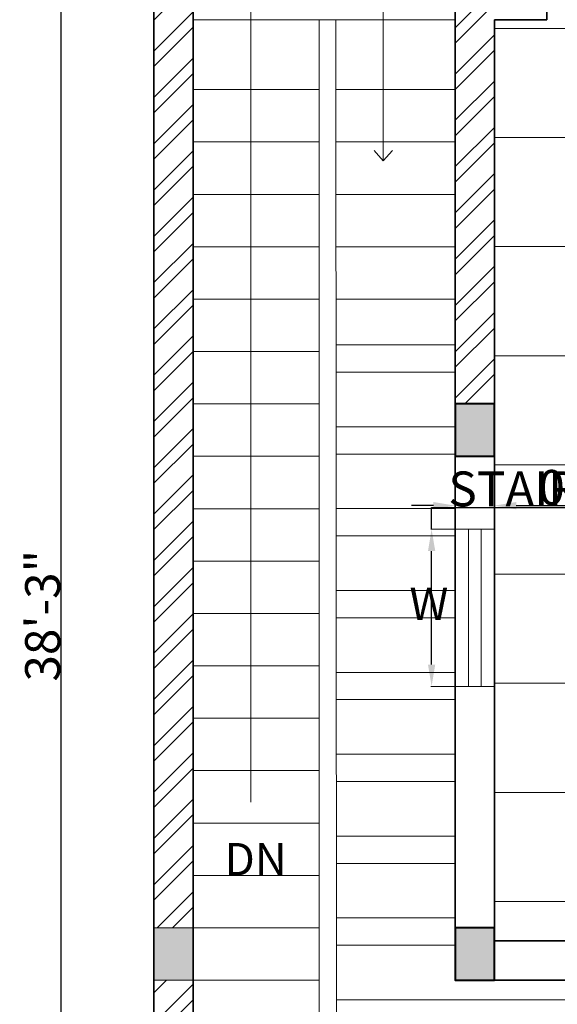
# Model space of a CAD drawing. Units: inches. Extents: x 351 to 1738, y -265 to 286.
# Tile 21 of 38: x 1004 to 1127, y -63 to 163. Entities that reach past the tile are written whole.
import ezdxf

# ---------------------------------------------------------------- set-up
doc = ezdxf.new("R2010")
doc.units = ezdxf.units.IN
doc.header["$MEASUREMENT"] = 0
for name, color, linetype, lineweight in [('A-ANNO-DIMS', 2, 'Continuous', 18), ('A-ANNO-SYMB', 7, 'Continuous', 18), ('A-COLS', 7, 'Continuous', 40), ('A-COLS-PATT', 6, 'Continuous', 13), ('A-FLOR-PATT', 9, 'Continuous', 9), ('A-FLOR-STRS', 7, 'Continuous', 18), ('A-GLAZ', 4, 'Continuous', 18), ('A-WALL', 7, 'Continuous', 35), ('A-WALL-PATT', 152, 'Continuous', 13)]:
    doc.layers.add(name, color=color, linetype=linetype, lineweight=lineweight)
doc.styles.add('Annotative', font='arial.ttf')
doc.styles.get("Standard").update_dxf_attribs({"font": 'arial.ttf'})
doc.dimstyles.get("Standard").update_dxf_attribs({"dimtxt": 8, "dimasz": 5, "dimexe": 0.18, "dimexo": 0.0625, "dimgap": 0.09, "dimtad": 1, "dimtoh": 1, "dimzin": 0, "dimdsep": 46, "dimlunit": 4, "dimtxsty": 'Standard', "dimcen": 0, "dimclre": 256, "dimadec": 0, "dimazin": 0, "dimtfac": 1, "dimtofl": 0, "dimtmove": 0, "dimatfit": 3, "dimfxl": 1, "dimtolj": 1, "dimtzin": 0, "dimlwe": -1, "dimarcsym": 0})

# ---------------------------------------------------------------- blocks, each defined once
blk = doc.blocks.new('*D8')
at = {"layer": 'A-ANNO-DIMS', "color": 0, "transparency": 16777216}
for p, q in [((1034.64, 255.96), (1013.22, 255.96)), ((1034.64, -203.04), (1013.22, -203.04))]:
    blk.add_line(p, q, dxfattribs=at)
at = {"layer": 'A-ANNO-DIMS', "color": 0, "lineweight": -2, "transparency": 16777216}
blk.add_line((1013.4, 250.96), (1013.4, -198.04), dxfattribs=at)
at = {"layer": 'A-ANNO-DIMS', "color": 0, "transparency": 16777216}
for points in [[(1012.57, 250.96), (1014.23, 250.96), (1013.4, 255.96)], [(1012.57, -198.04), (1014.23, -198.04), (1013.4, -203.04)]]:
    blk.add_solid(points, dxfattribs=at)
at = {"layer": 'Defpoints', "color": 0, "transparency": 16777216}
for p in [(1034.7, 255.96), (1013.4, -203.04), (1034.7, -203.04)]:
    blk.add_point(p, dxfattribs=at)
at = {"layer": 'A-ANNO-DIMS', "color": 0, "transparency": 16777216, "insert": (1009.22, 26.46), "char_height": 8, "attachment_point": 5, "rotation": 90}
blk.add_mtext('\\A1;38\'-3"', dxfattribs=at)
blk = doc.blocks.new('COL-9x12')
blk.add_lwpolyline([(0, 12), (0, 0), (9, 0), (9, 12)], close=True)
blk = doc.blocks.new('WIN-36-STAIR')
for p, q in [((3.02, 0), (3.02, 36)), ((5.92, 0), (5.92, 36))]:
    blk.add_line(p, q)
blk.add_lwpolyline([(0, 0), (0, 36), (9, 36), (9, 0)], close=True)
blk = doc.blocks.new('*D52')
at = {"layer": 'A-ANNO-DIMS', "color": 0, "lineweight": -2, "transparency": 16777216}
for p, q in [((1098.3, 46.26), (1098.3, 51.26)), ((1098.3, 51.26), (1235.28, 51.26)), ((1098.3, 15.26), (1098.3, 41.26))]:
    blk.add_line(p, q, dxfattribs=at)
at = {"layer": 'A-ANNO-DIMS', "transparency": 16777216}
for p, q in [((1103.64, 46.26), (1098.12, 46.26)), ((1103.64, 10.26), (1098.12, 10.26))]:
    blk.add_line(p, q, dxfattribs=at)
at = {"layer": 'A-ANNO-DIMS', "color": 0, "transparency": 16777216}
for points in [[(1097.47, 41.26), (1099.14, 41.26), (1098.3, 46.26)], [(1097.47, 15.26), (1099.14, 15.26), (1098.3, 10.26)]]:
    blk.add_solid(points, dxfattribs=at)
at = {"layer": 'Defpoints', "color": 0, "transparency": 16777216}
for p in [(1098.3, 46.26), (1103.7, 46.26), (1103.7, 10.26)]:
    blk.add_point(p, dxfattribs=at)
at = {"layer": 'A-ANNO-DIMS', "color": 0, "transparency": 16777216, "insert": (1166.84, 55.49), "char_height": 8, "attachment_point": 5}
blk.add_mtext('\\A1;STAIR WINDOW 3\'-0" TYP.', dxfattribs=at)
blk = doc.blocks.new('*D53')
at = {"layer": 'A-ANNO-DIMS', "color": 0, "lineweight": -2, "transparency": 16777216}
for p, q in [((1098.7, 51.66), (1093.7, 51.66)), ((1117.7, 51.66), (1171.65, 51.66))]:
    blk.add_line(p, q, dxfattribs=at)
at = {"layer": 'A-ANNO-DIMS', "transparency": 16777216}
for p, q in [((1103.7, 46.32), (1103.7, 51.84)), ((1112.7, 46.32), (1112.7, 51.84))]:
    blk.add_line(p, q, dxfattribs=at)
at = {"layer": 'A-ANNO-DIMS', "color": 0, "transparency": 16777216}
for points in [[(1098.7, 52.49), (1098.7, 50.82), (1103.7, 51.66)], [(1117.7, 52.49), (1117.7, 50.82), (1112.7, 51.66)]]:
    blk.add_solid(points, dxfattribs=at)
at = {"layer": 'Defpoints', "color": 0, "transparency": 16777216}
for p in [(1112.7, 51.66), (1103.7, 46.26), (1112.7, 46.26)]:
    blk.add_point(p, dxfattribs=at)
at = {"layer": 'A-ANNO-DIMS', "color": 0, "transparency": 16777216, "insert": (1147.18, 55.83), "char_height": 8, "attachment_point": 5}
blk.add_mtext('\\A1;0\'-9" TYP.', dxfattribs=at)

msp = doc.modelspace()

# ---------------------------------------------------------------- hatches: boundary and pattern name
at = {"layer": 'A-COLS-PATT'}
h = msp.add_hatch(color=256, dxfattribs=at)
h.dxf.hatch_style = 1
h.paths.add_polyline_path([(1112.704, 237.963), (1103.704, 237.963), (1103.704, 228.963), (1112.704, 228.963)])
h.paths.add_polyline_path([(1115.704, 237.963), (1112.704, 237.963), (1112.704, 228.963), (1115.704, 228.963)])
h.paths.add_polyline_path([(1043.704, 255.963), (1034.704, 255.963), (1034.704, 243.963), (1043.704, 243.963)])
h.paths.add_polyline_path([(1043.704, 210.963), (1034.704, 210.963), (1034.704, 198.963), (1043.704, 198.963)])
h.paths.add_polyline_path([(1043.704, -45.037), (1034.704, -45.037), (1034.704, -57.037), (1043.704, -57.037)])
h.paths.add_polyline_path([(1112.704, -45.037), (1103.704, -45.037), (1103.704, -57.037), (1112.704, -57.037)])
h.paths.add_polyline_path([(1112.704, -161.037), (1103.704, -161.037), (1103.704, -164.037), (1103.704, -173.037), (1112.704, -173.037)])
h.paths.add_polyline_path([(1043.704, -161.037), (1034.704, -161.037), (1034.704, -173.037), (1043.704, -173.037)])
h.paths.add_polyline_path([(1248.549, -164.037), (1236.549, -164.037), (1236.549, -173.037), (1248.549, -173.037)])
h.paths.add_polyline_path([(1248.549, -50), (1236.549, -50), (1236.549, -59), (1248.549, -59)])
h.paths.add_polyline_path([(1248.704, 73.463), (1244.704, 73.463), (1244.704, 64.463), (1248.704, 64.463)])
h.paths.add_polyline_path([(1244.704, 73.463), (1236.704, 73.463), (1236.704, 64.463), (1244.704, 64.463)])
h.paths.add_polyline_path([(1248.704, 237.963), (1236.704, 237.963), (1236.704, 228.963), (1248.704, 228.963)])
h.paths.add_polyline_path([(1392.204, 237.963), (1380.204, 237.963), (1380.204, 228.963), (1392.204, 228.963)])
h.paths.add_polyline_path([(1536.064, 237.963), (1524.064, 237.963), (1524.064, 228.963), (1536.064, 228.963)])
h.paths.add_polyline_path([(1536.064, 73.463), (1524.064, 73.463), (1524.064, 64.463), (1536.064, 64.463)])
h.paths.add_polyline_path([(1384.204, 73.463), (1380.204, 73.463), (1380.204, 64.463), (1384.204, 64.463)])
h.paths.add_polyline_path([(1392.064, 73.463), (1384.204, 73.463), (1384.204, 64.463), (1392.064, 64.463)])
h.paths.add_polyline_path([(1536.064, -53.037), (1524.064, -53.037), (1524.064, -57.037), (1536.064, -57.037)])
h.paths.add_polyline_path([(1536.064, -48.037), (1524.064, -48.037), (1524.064, -53.037), (1536.064, -53.037)])
h.paths.add_polyline_path([(1392.064, -48.037), (1380.064, -48.037), (1380.064, -56.5), (1380.065, -57.037), (1392.064, -57.037)])
h.paths.add_polyline_path([(1536.064, -164.037), (1524.064, -164.037), (1524.064, -173.037), (1536.064, -173.037)])
h = msp.add_hatch(color=256, dxfattribs=at)
h.dxf.hatch_style = 1
h.paths.add_polyline_path([(1112.704, 74.963), (1103.704, 74.963), (1103.704, 62.963), (1112.704, 62.963)])
at = {"layer": 'A-FLOR-PATT', "transparency": 33554559}
h = msp.add_hatch(dxfattribs=at)
h.set_pattern_fill('ANSI37', color=256, scale=200, angle=135)
h.set_pattern_definition([(180, (1112.704, -164.037), (-2e-15, -25), []), (270, (1112.704, -164.037), (25, -5e-15), [])])
h.paths.add_polyline_path([(1380.064, 73.463), (1380.132, 148.463), (1338.064, 148.463), (1290.704, 148.463), (1290.704, 88.463), (1248.704, 88.463), (1248.704, -2.009), (1244.704, -2.009), (1244.704, 142.457), (1160.704, 142.457), (1160.704, 158.963), (1160.704, 170.137), (1160.704, 206.137), (1160.704, 228.963), (1112.704, 228.963), (1112.704, 209.963), (1112.704, 168.963), (1124.704, 168.963), (1124.704, 162.963), (1112.704, 162.963), (1112.704, 64.463), (1112.704, 60.463), (1112.704, 0.463), (1112.704, -48.026), (1146.804, -47.981), (1146.804, -35.691), (1207.804, -35.691), (1207.804, -47.902), (1236.542, -47.864), (1236.544, -50.009), (1248.5, -50.009), (1248.506, -102.915), (1248.512, -150.915), (1248.514, -164.037), (1248.549, -164.037), (1273.017, -164.037), (1273.017, -128.799), (1355.24, -128.799), (1355.24, -164.037), (1384.204, -164.037), (1384.204, -57.037), (1380.064, -57.037), (1380.064, -48.037), (1392.064, -48.037), (1392.064, -53.037), (1406.549, -53.037), (1406.549, -57.037), (1401.204, -57.037), (1401.204, -147.037), (1468.204, -147.037), (1468.204, -138.5), (1472.204, -138.5), (1472.204, -102.5), (1468.204, -102.5), (1468.204, -57.037), (1442.549, -57.037), (1442.549, -53.037), (1463.049, -53.037), (1463.049, -40.747), (1524.049, -40.747), (1524.049, -48.037), (1536.064, -48.037), (1536.064, -53.037), (1557.704, -53.037), (1557.704, 204.963), (1384.204, 204.963), (1384.204, 73.463), (1392.064, 73.463), (1392.064, 64.463), (1384.204, 64.463), (1384.204, -3.5), (1380.204, -3.537), (1380.204, 64.463), (1380.064, 64.463)])
h.paths.add_polyline_path([(1510.714, 86.458, -0.1039845), (1511.661, 85.595, 0.4704384), (1510.158, 87.614, 0.0961001)], flags=16)
h.paths.add_polyline_path([(1510.443, 100.266, 0.009798), (1504.693, 100.48, 0.0287898), (1504.6, 99.767, -0.1653311), (1505.519, 96.135, -0.1436014)], flags=16)
h.paths.add_polyline_path([(1487.201, 85.595, -0.1039845), (1488.148, 86.458, 0.0961001), (1488.704, 87.614, 0.4704384)], flags=0)
h.paths.add_polyline_path([(1495.052, 100.43), (1494.178, 100.43, -0.0264629), (1494.262, 99.774, -0.1442193)], flags=16)
h.paths.add_polyline_path([(1444.485, 86.458, -0.1039845), (1445.433, 85.595, 0.4704384), (1443.93, 87.614, 0.0961001)], flags=16)
h.paths.add_polyline_path([(1420.972, 85.595, -0.1039845), (1421.92, 86.458, 0.0961001), (1422.475, 87.614, 0.4704384)], flags=16)
h.paths.add_polyline_path([(1428.632, 100.335, 0.0010541), (1427.971, 100.309, -0.0215241), (1428.033, 99.774, -0.1143008)], flags=16)
h.paths.add_polyline_path([(1419.906, 143.708, 0.0249793), (1420.222, 157.526), (1421.573, 159.101), (1421.573, 175.369), (1391.393, 175.369), (1391.393, 200.519), (1542.294, 200.519), (1542.294, 175.369), (1512.028, 175.369, 0.0198653), (1511.521, 153.838, 0.0251335), (1512.758, 118.323, 0.0205529), (1512.942, 115.253), (1419.834, 115.253, -0.0004142), (1419.843, 124.798), (1413.059, 124.798), (1413.059, 84.437, -0.0618528), (1415.831, 80.45, -0.0930773), (1420.972, 85.595, -0.2675367), (1422.371, 84.732, 0.0851103), (1424.052, 84.616, -0.8853927), (1424.033, 84.851, -1.1258145), (1424.073, 84.366, -0.0879871), (1422.371, 84.732, -0.2675367), (1422.326, 83.089, -0.3705421), (1420.972, 85.595, 0.0930773), (1415.831, 80.45, -0.0874142), (1417.914, 73.937), (1418.941, 73.937, 0.0272504), (1418.913, 76.906, -0.1157032), (1421.051, 73.937), (1445.354, 73.937, -0.1157032), (1447.492, 76.906, 0.0272504), (1447.464, 73.937), (1448.491, 73.937, -0.0874142), (1450.574, 80.45, 0.0930773), (1445.433, 85.595, -0.3705421), (1444.079, 83.089, -0.2675367), (1444.034, 84.732, -0.0879871), (1442.332, 84.366, -1.1258145), (1442.372, 84.851, -2.0327363), (1442.364, 84.368, 0.0863779), (1444.034, 84.732, -0.2675367), (1445.433, 85.595, -0.0930773), (1450.574, 80.45, -0.2577317), (1466.483, 90.927, -0.4786702), (1468.832, 91.907, -0.4786702), (1471.18, 90.927, -0.26264), (1483.053, 81.78, -0.0718662), (1487.201, 85.595, -0.2675367), (1488.6, 84.732, 0.0851103), (1490.28, 84.616, -0.8853927), (1490.262, 84.851, -1.1258145), (1490.301, 84.366, -0.0879871), (1488.6, 84.732, -0.2675367), (1488.554, 83.089, -0.3705421), (1487.201, 85.595, 0.0718662), (1483.053, 81.78, -0.1320648), (1484.143, 73.937), (1485.169, 73.937, 0.0272504), (1485.142, 76.906, -0.1157032), (1487.28, 73.937), (1511.582, 73.937, -0.1157032), (1513.72, 76.906, 0.0272504), (1513.693, 73.937), (1514.719, 73.937, -0.0874142), (1516.802, 80.45, 0.0930773), (1511.661, 85.595, -0.3705421), (1510.308, 83.089, -0.2675367), (1510.262, 84.732, -0.0879871), (1508.561, 84.366, -1.1258145), (1508.601, 84.851, -2.0327363), (1508.592, 84.368, 0.0863779), (1510.262, 84.732, -0.2675367), (1511.661, 85.595, -0.0930773), (1516.802, 80.45, -0.0618528), (1519.575, 84.437), (1519.575, 73.937), (1413.059, 73.937), (1413.059, 124.798), (1419.843, 124.798, -0.0008205)], flags=16)
h.paths.add_polyline_path([(1220.149, 54.133, -0.1039845), (1220.869, 53.476, 0.4704384), (1219.727, 55.011, 0.0961001)], flags=16)
h.paths.add_polyline_path([(1219.944, 64.626, 0.009798), (1215.574, 64.789, 0.0287898), (1215.503, 64.247, -0.1653311), (1216.201, 61.487, -0.1436014)], flags=16)
h.paths.add_polyline_path([(1209.779, 64.449, 0.0974459), (1209.339, 64.751), (1208.247, 64.751, 0.1273905), (1207.7, 64.326, 0.1715858), (1206.95, 61.475, -0.1588542), (1207.636, 59.45, 0.0158984), (1207.795, 59.218, 0.0615457), (1208.598, 59.616, 0.1754158), (1208.638, 60.099, -0.2847793), (1209.348, 62.472, 0.3262165)], flags=16)
h.paths.add_polyline_path([(1169.818, 54.133, -0.1039845), (1170.538, 53.476, 0.4704384), (1169.396, 55.011, 0.0961001)], flags=16)
h.paths.add_polyline_path([(1159.017, 62.472, 0.2847642), (1158.307, 60.099, -0.1754332), (1158.267, 59.616, 0.3929302), (1159.448, 64.449, -0.3262298)], flags=16)
h.paths.add_polyline_path([(1156.342, 58.239, -0.1783213), (1154.011, 55.31, -0.1747359), (1154.722, 55.233, -0.2008015), (1156.27, 56.086, 0.1269899), (1157.283, 58.991, -0.0912053)], flags=16)
h.paths.add_polyline_path([(1156.624, 61.413, 0.1572752), (1157.316, 64.247, 0.1696217)], flags=16)
h.paths.add_polyline_path([(1152.67, 54.133, -0.0961001), (1151.95, 53.476, 0.0640762), (1154.465, 54.384, 0.1990158)], flags=16)
h.paths.add_polyline_path([(1202.281, 53.476, -0.1039845), (1203, 54.133, 0.0961001), (1203.423, 55.011, 0.4704384)], flags=0)
h.paths.add_polyline_path([(1151.139, 97.64, 0.0249793), (1151.379, 108.141), (1152.406, 109.338), (1152.406, 121.701), (1129.47, 121.701), (1129.47, 140.814), (1244.149, 140.814), (1244.149, 121.701), (1221.148, 121.701, 0.0198653), (1220.763, 105.338, 0.0251335), (1221.703, 78.349, 0.0205529), (1221.843, 76.016), (1151.078, 76.016, -0.1287433), (1148.786, 65.037, 0.5393525), (1150.327, 64.171, -0.027594), (1163.481, 64.751, 0.0976954), (1163.04, 64.449, 0.3262165), (1163.471, 62.472, -0.2847765), (1164.181, 60.099, -0.1947567), (1165.846, 61.443, -0.1554021), (1165.172, 64.247, -0.1660224), (1165.869, 61.475, -0.1770142), (1167.852, 62.77, -0.4482027), (1169.974, 60.807, -0.3934987), (1167.679, 57.86, -0.8955483), (1168.438, 54.524, -0.3557668), (1166.218, 56.086, -0.066024), (1165.505, 57.539), (1165.251, 56.243, -0.3717324), (1164.02, 59.758, -0.3736141), (1163.04, 64.449, -0.0976954), (1163.481, 64.751, 0.0213538), (1153.294, 64.429, -0.1341826), (1156.695, 61.368, 0.1868727), (1154.636, 62.77, 0.4482027), (1152.514, 60.807, 0.4037263), (1154.905, 57.846, 0.7112192), (1153.334, 55, 0.5315397), (1151.95, 53.476, -0.2675367), (1153.013, 52.821, 0.0851103), (1154.29, 52.732, -0.8853927), (1154.276, 52.911, -1.1258145), (1154.306, 52.543, -0.0879871), (1153.013, 52.821, -0.2675367), (1152.978, 51.572, -0.3705421), (1151.95, 53.476, 0.0930773), (1148.043, 49.566, -0.0874142), (1149.626, 44.617), (1150.406, 44.617, 0.0272504), (1150.385, 46.873, -0.1157032), (1152.01, 44.617), (1170.478, 44.617, -0.1157032), (1172.103, 46.873, 0.0272504), (1172.082, 44.617), (1172.862, 44.617, -0.0874142), (1174.445, 49.566, 0.0930773), (1170.538, 53.476, -0.3705421), (1169.51, 51.572, -0.2675367), (1169.475, 52.821, -0.0879871), (1168.182, 52.543, -1.1258145), (1168.212, 52.911, -2.0327363), (1168.206, 52.544, 0.0863779), (1169.475, 52.821, -0.2675367), (1170.538, 53.476, -0.0930773), (1174.445, 49.566, -0.2577317), (1186.536, 57.528, -0.4786702), (1188.321, 58.273, -0.4786702), (1190.106, 57.528, -0.26264), (1199.128, 50.577, -0.0718662), (1202.281, 53.476, -0.2675367), (1203.344, 52.821, 0.0851103), (1204.621, 52.732, -0.8853927), (1204.607, 52.911, -1.1258145), (1204.637, 52.543, -0.0879871), (1203.344, 52.821, -0.2675367), (1203.309, 51.572, -0.3705421), (1202.281, 53.476, 0.0718662), (1199.128, 50.577, -0.1320648), (1199.957, 44.617), (1200.737, 44.617, 0.0272504), (1200.716, 46.873, -0.1157032), (1202.341, 44.617), (1220.809, 44.617, -0.1157032), (1222.434, 46.873, 0.0272504), (1222.413, 44.617), (1223.193, 44.617, -0.0874142), (1224.776, 49.566, 0.0930773), (1220.869, 53.476, -0.3705421), (1219.841, 51.572, -0.2675367), (1219.806, 52.821, -0.0879871), (1218.513, 52.543, -1.1258145), (1218.543, 52.911, -2.0327363), (1218.537, 52.544, 0.0863779), (1219.806, 52.821, -0.2675367), (1220.869, 53.476, -0.0930773), (1224.776, 49.566, -0.0618528), (1226.883, 52.597), (1226.883, 44.617), (1145.936, 44.617), (1145.936, 83.269), (1151.091, 83.269, -0.0008205)], flags=16)
h.paths.add_polyline_path([(1218.01, 57.86, -0.8955483), (1218.769, 54.524, -0.3557668), (1216.549, 56.086, -0.066024), (1215.836, 57.539), (1215.582, 56.243, -0.3717324), (1214.351, 59.758, -0.3736141), (1213.371, 64.449, 0.3262165), (1213.802, 62.472, -0.2847765), (1214.512, 60.099, -0.1947567), (1216.177, 61.443, -0.1799907), (1218.183, 62.77, -0.4482027), (1220.305, 60.807, -0.3934987)], flags=16)
h.paths.add_polyline_path([(1424.735, 91.363, -0.3934987), (1421.715, 95.241, -0.4482027), (1424.507, 97.824, -0.1799907), (1427.147, 96.077, -0.1947567), (1429.338, 94.309, -0.2847765), (1430.272, 97.432, 0.3262165), (1430.839, 100.034, -0.3736141), (1429.55, 93.861, -0.3717324), (1427.929, 89.235), (1427.596, 90.941, -0.066024), (1426.657, 89.029, -0.3557668), (1423.736, 86.973, -0.8955483)], flags=16)
h.paths.add_polyline_path([(1238.033, 131.257, -1), (1227.329, 131.257, -1)], flags=0)
h.paths.add_polyline_path([(1235.357, 131.257, -1), (1230.005, 131.257, -1)], flags=0)
h.paths.add_polyline_path([(1214.039, 54.243, 0.1543819), (1214.38, 53.992, 0.3589549), (1213.613, 54.016, 0.6039484), (1214.379, 53.657, 0.3713191), (1213.968, 52.872, 0.1879935), (1214.312, 52.809, -0.592455), (1213.953, 52.967, -0.2942791), (1214.083, 53.691, -1.3001871), (1213.881, 54.134, -0.2837621), (1214.469, 53.896, 1.1509396)], flags=16)
h.paths.add_polyline_path([(1212.091, 56.286, -0.4084338), (1211.337, 56.445, -0.0362594), (1211.098, 56.848, -0.2360976), (1211.59, 56.63, 0.0353445), (1211.835, 56.543, -0.4752408), (1212.091, 56.286, -0.4752408), (1212.438, 56.182, 0.0353445), (1212.631, 56.007, -0.2360976), (1213.056, 55.676, -0.0362594), (1212.588, 55.697, -0.4084338)], flags=16)
h.paths.add_polyline_path([(1211.469, 50.297, 0.296043), (1210.47, 50.527, 0.310883), (1211.931, 50.148, 0.0212546)], flags=16)
h.paths.add_polyline_path([(1213.739, 51.818, -0.0362594), (1213.271, 51.838, -0.4084337), (1212.774, 52.427, -0.0947856), (1212.293, 50.703, 1.1504738), (1212.911, 50.232, 0.1662877), (1213.265, 50.68, -0.0252543), (1212.603, 50.13, 1.0879317), (1212.471, 49.407, 0.1662877), (1213.02, 49.251, -0.016128), (1212.567, 49.563, -0.286859), (1212.217, 49.638, 0.0221563), (1212.046, 50.055, -0.6461302), (1212.185, 50.498, 0.0884116), (1212.732, 52.077, -1.1860374), (1213.121, 52.323, 0.0353445), (1213.314, 52.148, -0.2360976)], flags=16)
h.paths.add_polyline_path([(1212.094, 50.342, -0.0485241), (1211.54, 49.605, -1.1038339), (1211.397, 48.738, -0.7855147), (1211.683, 48.254, -0.3920429), (1210.948, 48.525, -0.3928194), (1210.561, 47.995, -0.592455), (1210.201, 48.153, -0.2942791), (1210.331, 48.877, -0.7041716), (1210.316, 49.592, -0.6793441), (1210.729, 50.112, 0.5636764)], flags=16)
h.paths.add_polyline_path([(1211.274, 49.829, -0.1398258), (1210.745, 49.859, -0.2178785), (1210.948, 49.509, -0.4985724)], flags=0)
h.paths.add_polyline_path([(1433.426, 81.49, -0.181571), (1434.245, 81.788, -0.0080665), (1433.726, 82.205, 0.0455784), (1432.755, 81.242, 0.1790113)], flags=16)
h.paths.add_polyline_path([(1434.146, 81.009, -0.1324418), (1433.645, 80.771, 0.2590893), (1433.234, 80.471, -0.1802109), (1433.392, 80.805, -0.1699398), (1432.758, 81.109, 0.0326525), (1433.273, 80.474, -0.4933627), (1434.046, 80.146, -0.3904966)], flags=16)
h.paths.add_polyline_path([(1434.83, 80.047, -0.9475376), (1435.294, 79.576, -0.2991282), (1434.625, 79.404, -0.2704392), (1435.01, 78.591, -0.592455), (1434.537, 78.382, -0.3928194), (1434.027, 79.08, -0.3920429), (1433.06, 78.723, -0.3520423), (1433.003, 79.197, -0.1972159), (1433.75, 79.734, -0.7136405), (1434.447, 79.939, -0.2147903), (1434.819, 80.475, 0.4088333), (1435.075, 80.803, -0.2261519)], flags=16)
h.paths.add_polyline_path([(1432.67, 81.217, -0.4542182), (1431.897, 79.923, -0.4144105), (1431.301, 80.035, 0.0161291), (1431.897, 80.445, 0.2795702), (1432.073, 80.871, -0.2895037), (1431.103, 81.321, -0.4144105), (1430.978, 81.915, 0.0161296), (1431.586, 81.521, 0.341293), (1432.125, 81.583, -0.8131856)], flags=16)
h.paths.add_polyline_path([(1429.893, 86.381, -0.9475376), (1430.358, 85.91, -0.1731062), (1429.984, 85.712, -0.0388172), (1431.625, 84.214, -0.0879005), (1432.097, 88.549, -0.0497684), (1431.254, 88.49, -0.2360976), (1431.814, 88.925, 0.0353445), (1432.067, 89.155, -0.4752408), (1432.524, 89.291, -0.4752408), (1432.86, 89.63, 0.0353445), (1433.182, 89.744, -0.2360976), (1433.83, 90.032, -0.0362594), (1433.516, 89.502, -0.4084338), (1432.524, 89.291, -0.3124239), (1432.106, 88.58, 0.0885594), (1431.625, 84.214, -0.4084337), (1430.971, 83.439, -0.0362594), (1430.355, 83.412, -0.2360976), (1430.914, 83.847, 0.0353445), (1431.168, 84.078, -0.4752408), (1431.625, 84.214, 0.0388172), (1429.984, 85.712, -0.3217316), (1429.333, 86.048, -0.32743), (1429.883, 86.809, 0.4088333), (1430.138, 87.138, -0.2261519)], flags=16)
h.paths.add_polyline_path([(1211.206, 58.616, -0.9997836), (1211.336, 59.323, -0.6149935)], flags=16)
h.paths.add_polyline_path([(1210.288, 49.429, 0.1543819), (1210.629, 49.178, 0.3589549), (1209.861, 49.202, 0.6039484), (1210.627, 48.843, -0.5348247), (1210.806, 49.295, 0.7483464)], flags=16)
h.paths.add_polyline_path([(1209.589, 51.828, -0.0087906), (1209.775, 51.753, 0.1122315), (1209.466, 52.019, 1.4188509), (1209.014, 51.708, -0.4587257), (1208.651, 51.073, -0.592455), (1208.291, 51.232, -0.2942791), (1208.421, 51.955, -1.3001871), (1208.219, 52.398, -0.2260052), (1208.719, 52.257, -0.4755189), (1209.158, 52.369, -1.4554994), (1209.603, 52.664, 0.4213049), (1209.191, 52.262, -0.5912116), (1208.979, 51.796, 0.4973986), (1209.773, 51.333, 0.6493116)], flags=16)
h.paths.add_polyline_path([(1208.029, 52.041, 0.5446671), (1208.832, 52.045, 0.220132)], flags=0)
h.paths.add_polyline_path([(1210.438, 51.425, -0.2041997), (1210.277, 52.018, 0.2708262), (1209.915, 52.897, 0.3241145)], flags=0)
h.paths.add_polyline_path([(1209.668, 52.407, -0.60139), (1208.99, 52.221, -0.3949159), (1208.248, 52.83, -0.8367916), (1208.651, 53.017, -0.3384876), (1209.039, 52.571, 0.1941379), (1209.191, 52.262, 0.4139945), (1209.712, 52.475, 0.5177103), (1210.503, 51.416, 0.401922), (1209.493, 50.93, 0.2063956), (1209.516, 50.165, -0.3194629), (1210.417, 51.418, -0.466635)], flags=16)
h.paths.add_polyline_path([(1206.601, 56.086, -0.3557668), (1204.381, 54.524, -0.9211983), (1205.236, 57.846, 0.2065693), (1207.614, 58.991, -0.1269899)], flags=16)
h.paths.add_polyline_path([(1435.487, 82.816, 0.5277653), (1436.615, 83.361, 0.5085402), (1437.05, 82.433, 0.592455), (1437.524, 82.641, 0.3312448), (1436.963, 83.548, 0.3878632), (1437.808, 83.626, 0.5929544), (1437.618, 84.176, 0.2260158), (1436.961, 83.99, 0.3182053), (1437.588, 84.854, 0.6893744), (1437.05, 84.991, 0.3357648), (1436.539, 84.41, -0.1569934), (1436.404, 84.065, -0.4346112), (1436.961, 83.99, -0.2147903), (1437.333, 84.526, 0.4088333), (1437.588, 84.854, -0.2261519), (1437.343, 84.097, -0.9475376), (1437.808, 83.626, -0.2991282), (1437.139, 83.455, -0.2704392), (1437.524, 82.641, -0.592455), (1437.05, 82.433, -0.3928194), (1436.541, 83.13, -0.4396601), (1435.475, 82.794, -0.174614), (1435.942, 82.244, -0.2063956), (1435.912, 81.237, -0.2708262), (1435.125, 82.208, 0.2079765), (1434.686, 82.904, -0.1964955)], flags=16)
h.paths.add_polyline_path([(1435.386, 84.832, 0.270811), (1434.91, 83.676, -0.2042174), (1434.699, 82.895, 0.3241145)], flags=0)
h.paths.add_polyline_path([(1435.68, 84.18, -0.2176564), (1435.554, 83.304, -0.1767045), (1436.236, 83.778, -0.3730364)], flags=0)
h.paths.add_polyline_path([(1435.566, 100.034, 0.3262165), (1436.133, 97.432, -0.2847765), (1437.067, 94.309, -0.1947567), (1439.258, 96.077, -0.1554021), (1438.371, 99.767, -0.1660224), (1439.289, 96.12, -0.1770142), (1441.897, 97.824, -0.4482027), (1444.69, 95.241, -0.3934987), (1441.67, 91.363, -0.8955483), (1442.669, 86.973, -0.3557668), (1439.748, 89.029, -0.066024), (1438.809, 90.941), (1438.476, 89.235, -0.3717324), (1436.855, 93.861, -0.3736141)], flags=16)
h.paths.add_polyline_path([(1191.252, 49.507, -0.2740221), (1190.658, 48.409, 0.2675367), (1191.311, 47.344, 0.3705421)], flags=0)
h.paths.add_polyline_path([(1190.301, 49.717, 0.1990158), (1188.619, 49.04, 0.0640762), (1191.252, 49.507, -0.0961001)], flags=0)
h.paths.add_polyline_path([(1189.518, 47.857, 1.1258145), (1189.676, 47.523, 2.0446052)], flags=0)
h.paths.add_polyline_path([(1464.974, 80.372, 0.2740221), (1465.756, 78.927, -0.0830131)], flags=0)
h.paths.add_polyline_path([(1464.974, 80.372, 0.3705421), (1464.897, 77.525, 0.5763244)], flags=0)
h.paths.add_polyline_path([(1464.974, 80.372, -0.4704384), (1467.284, 81.372, -0.0961001), (1466.226, 80.648, -0.1990158), (1468.439, 79.757, -0.0640762)], flags=0)
h.paths.add_polyline_path([(1189.511, 56.43, -0.2594668), (1188.321, 56.391, -0.2594668), (1187.13, 56.43, 0.0851103), (1188.193, 55.716, -0.8853927), (1188.27, 55.878, -1.1960133), (1188.355, 55.442, 0.1014587)], flags=0)
h.paths.add_polyline_path([(1188.321, 57.596, 0.0780722), (1187.678, 57.24, 0.0155503), (1188.321, 57.136, 0.0155503), (1188.964, 57.24, 0.0780722)], flags=0)
h.paths.add_polyline_path([(1190.164, 55.365, -0.5763244), (1190.106, 57.528, -0.1982945), (1188.321, 58.319, -0.1982945), (1186.536, 57.528, -0.5763244), (1186.477, 55.365, -0.3705421), (1186.536, 57.528, 0.1982945), (1188.321, 58.319, 0.1982945), (1190.106, 57.528, -0.3705421)], flags=0)
h.paths.add_polyline_path([(1188.372, 55.878, 1.1258145), (1188.529, 55.544, 2.0446052)], flags=0)
h.paths.add_polyline_path([(1186.341, 49.717, -0.0961001), (1185.389, 49.507, 0.0640762), (1188.022, 49.04, 0.1990158)], flags=0)
h.paths.add_polyline_path([(1185.389, 49.507, -0.2675367), (1185.984, 48.409, 0.0851103), (1187.046, 47.695, -0.8853927), (1187.123, 47.857, -1.1258145), (1186.966, 47.523, -0.0879871), (1185.984, 48.409, -0.2675367), (1185.331, 47.344, -0.3705421)], flags=0)
h.paths.add_polyline_path([(1399.441, 187.944, -1), (1413.525, 187.944, -1)], flags=0)
h.paths.add_polyline_path([(1402.962, 187.944, -1), (1410.004, 187.944, -1)], flags=0)
h.paths.add_polyline_path([(1357.663, -72.245), (1377.272, -72.245), (1377.272, -91.854), (1357.663, -91.854)], flags=16)
h.paths.add_polyline_path([(1467.256, 78.201, -1.1258145), (1467.049, 77.761, -2.0446052)], flags=0)
h.paths.add_polyline_path([(1468.822, 88.714, 0.9411249), (1469.106, 88.316, 1.1371523), (1468.765, 88.755, 0.890986), (1468.99, 88.245, 0.0948283), (1470.398, 89.481, -0.2675367), (1471.18, 90.927, -0.0281232), (1469.678, 90.547, -0.0287737), (1469.948, 90.311, -0.0203267), (1468.832, 90.41, -0.0203267), (1467.716, 90.311, -0.0287737), (1467.986, 90.547, -0.0281232), (1466.483, 90.927, -0.2675367), (1467.265, 89.481, 0.0851103), (1468.663, 88.542, -1.2023159)], flags=0)
h.paths.add_polyline_path([(1178.25, 124.523, -0.1199286), (1165.65, 124.145, -0.1073492), (1159.133, 124.446, -0.1028906), (1159.132, 130.465, -0.0748968), (1158.993, 137.956, 0.002027), (1167.844, 137.479, -0.07553), (1180.337, 137.666, -0.0758613), (1186.502, 137.688, -0.1409896), (1186.272, 130.046, -0.0954805), (1186.729, 124.748, -0.10603)], flags=0)
h.paths.add_polyline_path([(1469.225, 79.757, -0.1990158), (1471.437, 80.648, -0.0961001), (1470.379, 81.372, -0.4704384), (1472.689, 80.372, -0.3705421), (1472.766, 77.525, -0.2675367), (1471.907, 78.927, -0.0879863), (1470.615, 77.761, -1.1258491), (1470.408, 78.201, -2.0327363), (1470.642, 77.778, 0.0863779), (1471.907, 78.927, -0.2675367), (1472.689, 80.372, -0.0640762)], flags=0)
h.paths.add_polyline_path([(1430.423, 186.902, -0.0748968), (1430.24, 196.758, 0.002027), (1441.887, 196.131, -0.07553), (1458.326, 196.377, -0.0758613), (1466.438, 196.406, -0.1409896), (1466.136, 186.35, -0.0954805), (1466.737, 179.378, -0.10603), (1455.58, 179.082, -0.1199286), (1439, 178.585, -0.1073492), (1430.425, 178.981, -0.1028906)], flags=0)
h.paths.add_polyline_path([(1162.258, 49.939, 0.3357645), (1161.87, 49.497, -0.1569936), (1161.767, 49.235, -0.4346112), (1162.19, 49.178, -0.2147903), (1162.473, 49.585, 1.5291948)], flags=16)
h.paths.add_polyline_path([(1161.683, 49.021, 0.5815181), (1161.268, 49.583, 0.5927609)], flags=16)
h.paths.add_polyline_path([(1162.602, 48.058, 0.3713191), (1162.192, 48.843, 0.4345332), (1162.88, 48.962, 0.1850806), (1162.197, 48.926, 1.1218369)], flags=16)
h.paths.add_polyline_path([(1161.443, 48.941, -1.3071038), (1161.495, 48.571, -0.2177521), (1161.136, 48.254, 0.6973029), (1161.871, 49.048, 0.1215141)], flags=16)
h.paths.add_polyline_path([(1162.531, 49.429, -0.2070837), (1162.05, 49.146, -0.9920299)], flags=16)
h.paths.add_polyline_path([(1161.304, 49.578, -0.7196675), (1161.513, 50.079, -0.1304275), (1160.836, 50.168, 0.0395926)], flags=0)
h.paths.add_polyline_path([(1162.036, 50.584, -0.0080665), (1161.642, 50.9, 0.0293675), (1161.35, 50.297, -0.2057884)], flags=16)
h.paths.add_polyline_path([(1162.882, 51.392, -0.1247327), (1162.763, 51.828, -0.1011907), (1162.399, 51.438, -0.153425)], flags=0)
h.paths.add_polyline_path([(1164.235, 51.85, -0.3091075), (1164.513, 51.136, -0.6271245), (1163.781, 51.603, -0.6859091), (1162.777, 51.219, -0.2332851), (1163.303, 50.165, -0.2708262), (1162.705, 50.903, 0.2041997), (1162.381, 51.425, 0.204182), (1162.542, 52.018, -0.2708414), (1162.903, 52.897, -0.1272607), (1163.219, 52.529, -1.1686811), (1163.781, 52.587, -0.3291117), (1164.168, 53.017, -0.8367917), (1164.571, 52.83, -0.1933406), (1164.391, 52.338, -0.9475376), (1164.744, 51.981, -0.2991282)], flags=16)
h.paths.add_polyline_path([(1163.598, 51.937, -1.2629561), (1163.236, 51.831, 0.0125754), (1162.971, 51.721, 0.2306566), (1163.151, 52.407, -0.1648982), (1163.178, 52.661, -0.4493201), (1163.628, 52.262, -0.721477), (1164.154, 52.088, -0.8499982)], flags=0)
h.paths.add_polyline_path([(1161.613, 58.616, -0.9804131), (1161.525, 59.049, -2.9089348)], flags=16)
h.paths.add_polyline_path([(1160.252, 49.166, -0.4144105), (1159.799, 49.251, 0.0161291), (1160.252, 49.563, 0.2795702), (1160.386, 49.887, -0.2895037), (1159.649, 50.229, -0.4144105), (1159.554, 50.68, 0.0161296), (1160.015, 50.381, 0.6178854), (1160.526, 50.703, -0.0947856), (1160.045, 52.427, -0.1404436), (1159.682, 52.042, -0.0578559), (1159.3, 51.872, 0.5448433), (1160.046, 52.419, -0.0881216), (1160.404, 55.721, -0.0497684), (1159.763, 55.676, -0.2360976), (1160.188, 56.007, 0.0353445), (1160.381, 56.182, -0.4752408), (1160.728, 56.286, -0.4752408), (1160.984, 56.543, 0.0353445), (1161.229, 56.63, -0.2360976), (1161.721, 56.848, -0.0362594), (1161.482, 56.445, -0.4084338), (1160.728, 56.286, -0.3124239), (1160.411, 55.745, 0.0885594), (1160.045, 52.427, 0.1070813), (1160.634, 50.498, -0.4947977), (1160.839, 50.149, -0.4542182)], flags=16)
h.paths.add_polyline_path([(1160.666, 49.808, -2.0765276), (1160.828, 50.172, 0.0195861)], flags=0)
h.paths.add_polyline_path([(1158.439, 53.992, 0.1543819), (1158.78, 54.243, 0.7483463), (1158.262, 54.109, -0.3382251), (1158.492, 53.839, -0.1708158), (1159.124, 53.779, 0.4957286), (1158.938, 54.134, 0.2260157)], flags=16)
h.paths.add_polyline_path([(1160.045, 52.427, 0.0388172), (1158.798, 53.565, -0.1198178), (1158.574, 53.586, -0.3091075), (1158.851, 52.872, -0.1879935), (1158.506, 52.809, 0.592455), (1158.866, 52.967, 0.3312448), (1158.44, 53.657, 0.2012451), (1158.798, 53.565, -0.034023), (1159.901, 52.578, -0.0442527), (1159.698, 52.323, -0.4752408)], flags=16)
h.paths.add_polyline_path([(1336.926, -95.392), (1336.926, -117.945), (1291.82, -117.945), (1291.82, -95.392)], flags=16)
h.paths.add_polyline_path([(1357.535, -97.244), (1357.726, -96.697, 0.0348443)], flags=16)
h.paths.add_polyline_path([(1376.693, -96.478), (1377.301, -96.5, 0.0314968), (1375.907, -96.424), (1357.726, -96.424)], flags=16)
h.paths.add_polyline_path([(1379.403, -119.667, 0.0267056), (1380.043, -119.439, -0.0152991)], flags=16)
h.paths.add_polyline_path([(1357.726, -120.202), (1357.821, -120.202), (1357.821, -120.201)], flags=16)
h.paths.add_polyline_path([(1354.171, -104.592), (1354.469, -98.672, 0.0111377)], flags=16)
h.paths.add_polyline_path([(1355.058, -119.136), (1354.578, -118.539, 0.1431635)], flags=16)
h.paths.add_polyline_path([(1378.851, -96.821), (1378.85, -96.82), (1378.85, -96.82, -0.0496798), (1380.055, -97.191), (1378.85, -96.82, 0.1500541), (1375.135, -97.188), (1375.136, -119.44, -0.0099698), (1374.747, -116.649), (1357.726, -116.649, 0.1693849), (1357.535, -119.382), (1357.535, -119.382), (1357.535, -119.382, 0.0348176), (1357.726, -119.928), (1357.726, -119.928), (1357.726, -119.929, -0.0348772), (1357.535, -119.382), (1355.507, -119.382), (1355.317, -119.278), (1357.535, -119.382, -0.1693939), (1357.726, -116.649, -0.0391513), (1374.686, -116.113, -0.0020149), (1374.625, -115.546, 0.1153223), (1369.915, -115.474, 0.0609215), (1369.922, -101.154, 0.1151459), (1374.625, -101.079, -0.0020164), (1374.686, -100.513, -0.0391511), (1357.726, -99.977), (1374.747, -99.977, -0.0099633), (1375.135, -97.188), (1375.135, -97.188, -0.1501081)], flags=16)
h.paths.add_polyline_path([(1490.963, 91.363, -0.3934987), (1487.944, 95.241, -0.4482027), (1490.736, 97.824, -0.1799907), (1493.376, 96.077, -0.1947567), (1495.567, 94.309, -0.2847765), (1496.501, 97.432, 0.3262165), (1497.068, 100.034, -0.3736141), (1495.778, 93.861, -0.3717324), (1494.158, 89.235), (1493.824, 90.941, -0.066024), (1492.886, 89.029, -0.3557668), (1489.964, 86.973, -0.8955483)], flags=16)
h.paths.add_polyline_path([(1354.86, -97.658), (1355.316, -97.348, 0.1019112)], flags=16)
h.paths.add_polyline_path([(1497.063, 83.327, 0.1767244), (1496.37, 83.785, -0.4051388), (1496.016, 83.384, 0.4973986), (1497.06, 82.774, 0.6493116), (1496.818, 83.426, -0.0087906)], flags=16)
h.paths.add_polyline_path([(1496.339, 83.783, 0.5927609), (1496.886, 84.522, 0.5815181)], flags=16)
h.paths.add_polyline_path([(1495.11, 82.641, 0.592455), (1495.583, 82.433, 0.6769152), (1495.805, 83.59, 0.3756693)], flags=16)
h.paths.add_polyline_path([(1495.015, 84.176, -0.145057), (1495.301, 84.526, -0.4088333), (1495.045, 84.854, 0.2206292), (1495.381, 84.152, -0.199594), (1495.851, 83.764, -0.5240172), (1494.826, 83.626, -0.5929976)], flags=16)
h.paths.add_polyline_path([(1501.655, 81.915, -0.0161291), (1501.048, 81.521, -0.3927187), (1500.462, 81.37, -0.2106699), (1500.607, 81.142, 0.3066994)], flags=16)
h.paths.add_polyline_path([(1500.11, 89.291, -0.4084338), (1499.118, 89.502, -0.0362594), (1498.803, 90.032, -0.2360976), (1499.451, 89.744, 0.0353445), (1499.774, 89.63, -0.4752408), (1500.11, 89.291, -0.4752408), (1500.567, 89.155, 0.0353445), (1500.82, 88.925, -0.2360976), (1501.379, 88.49, -0.0362594), (1500.763, 88.516, -0.4084338)], flags=16)
h.paths.add_polyline_path([(1498.908, 82.205, -0.0513217), (1500.013, 81.134, -0.5879306), (1500.234, 81.676, 0.1070813), (1501.009, 84.214, -0.03529)], flags=16)
h.paths.add_polyline_path([(1496.93, 83.875, -0.2063956), (1497.247, 84.832, -0.2708262), (1497.724, 83.676, 0.2079765), (1497.944, 82.884, -0.3814554)], flags=16)
h.paths.add_polyline_path([(1496.721, 81.237, 0.2708125), (1497.509, 82.208, -0.2042157), (1497.935, 82.895, 0.3241145)], flags=16)
h.paths.add_polyline_path([(1497.529, 80.125, -0.145057), (1497.814, 80.475, -0.703182), (1498.282, 81.178, -0.1229248), (1497.977, 81.714, -0.2708368), (1499.207, 81.49, 0.2079641), (1499.993, 81.248, -0.2651454), (1499.278, 80.472, 0.3819006), (1498.808, 79.947, -0.3059049), (1498.848, 79.519, 0.4994816), (1498.574, 79.217, -0.4587257), (1498.097, 78.382, -0.592455), (1497.624, 78.591, -0.2704392), (1498.009, 79.404, -0.299116), (1497.34, 79.576, -0.5930157)], flags=16)
h.paths.add_polyline_path([(1500.736, 79.923, 0.4144105), (1501.333, 80.035, -0.3216484), (1500.192, 80.765, 0.0198856), (1499.976, 81.251, 0.4653307)], flags=16)
h.paths.add_polyline_path([(1501.009, 84.214, -0.0388172), (1502.649, 85.712, -0.1730946), (1502.276, 85.91, -0.5930157), (1502.465, 86.46, -0.145057), (1502.751, 86.809, -0.4088333), (1502.495, 87.138, 0.2206292), (1502.831, 86.436, -0.199594), (1503.301, 86.048, -0.3217316), (1502.649, 85.712, 0.0388172), (1501.009, 84.214, 0.1224486), (1501.412, 83.755, 0.4754908), (1501.335, 84.226, 0.055822), (1501.719, 83.847, -0.2360976), (1502.278, 83.412, -0.0362594), (1501.663, 83.439, -0.4084338)], flags=16)
h.paths.add_polyline_path([(1501.794, 100.034, 0.3262165), (1502.362, 97.432, -0.2847765), (1503.295, 94.309, -0.1947567), (1505.486, 96.077, -0.1799907), (1508.126, 97.824, -0.4482027), (1510.918, 95.241, -0.3934987), (1507.899, 91.363, -0.8955483), (1508.898, 86.973, -0.3557668), (1505.976, 89.029, -0.066024), (1505.038, 90.941), (1504.704, 89.235, -0.3717324), (1503.084, 93.861, -0.3736141)], flags=16)
h.paths.add_polyline_path([(1146.29, 131.257, -1), (1135.587, 131.257, -1)], flags=0)
h.paths.add_polyline_path([(1143.614, 131.257, -1), (1138.262, 131.257, -1)], flags=0)
h.paths.add_polyline_path([(1524.064, 73.463), (1536.064, 73.463), (1536.064, 64.463), (1524.064, 64.463)], flags=16)
h.paths.add_polyline_path([(1520.162, 187.944, -1), (1534.246, 187.944, -1)], flags=0)
h.paths.add_polyline_path([(1530.725, 187.944), (1527.204, 187.944), (1527.204, 184.423, 0.4142136)], flags=0)
h.paths.add_polyline_path([(1278.415, -91.154), (1331.067, -91.154), (1331.067, -80.583), (1278.415, -80.583)], flags=24)
h.paths.add_polyline_path([(1266.655, -79.354), (1354.738, -79.354), (1354.738, -67.817), (1266.655, -67.817)], flags=24)
h.paths.add_polyline_path([(1115.482, 206.184), (1155.098, 206.184), (1155.098, 217.714), (1115.482, 217.714)], flags=24)
h.paths.add_polyline_path([(1161.771, 8.501), (1222.466, 8.501), (1222.466, 19.079), (1161.771, 19.079)], flags=24)
h.paths.add_polyline_path([(1164.656, 18.795), (1210.615, 18.795), (1210.615, 30.324), (1164.656, 30.324)], flags=24)
h.paths.add_polyline_path([(1368.147, -32.882), (1379.362, -32.882), (1379.362, -21.733), (1368.147, -21.733)], flags=24)
h.paths.add_polyline_path([(1244.842, -31.012), (1256.057, -31.012), (1256.057, -19.863), (1244.842, -19.863)], flags=24)
h.paths.add_polyline_path([(1114.589, 195.739), (1156.517, 195.739), (1156.517, 206.31), (1114.589, 206.31)], flags=24)
h.paths.add_polyline_path([(1436.398, 37.632), (1505.131, 37.632), (1505.131, 48.203), (1436.398, 48.203)], flags=24)
h.paths.add_polyline_path([(1435.991, 47.919), (1507.906, 47.919), (1507.906, 59.456), (1435.991, 59.456)], flags=24)
h.paths.add_polyline_path([(1415.107, -124.896), (1457.038, -124.896), (1457.038, -114.318), (1415.107, -114.318)], flags=24)
h.paths.add_polyline_path([(1417.992, -114.602), (1457.609, -114.602), (1457.609, -103.073), (1417.992, -103.073)], flags=24)
h = msp.add_hatch(dxfattribs=at)
h.set_pattern_fill('ANSI32', color=256, scale=50, angle=135)
h.set_pattern_definition([(180, (1038.704, -199.037), (-2e-15, -18.75), []), (180, (1032.454, -192.787), (-2e-15, -18.75), [])])
h.paths.add_polyline_path([(1248.506, -102.915), (1236.559, -102.916), (1236.553, -56.864), (1112.704, -57.026), (1112.704, -57.037), (1103.704, -57.037), (1103.704, -45.037), (1103.704, 98.963), (1076.434, 98.963), (1076.549, -81.037), (1071.549, -81.037), (1043.704, -81.037), (1038.704, -81.037), (1038.704, -161.037), (1043.704, -161.037), (1043.704, -173.037), (1038.704, -173.037), (1038.704, -199.037), (1562.704, -199.037), (1562.704, -173.037), (1236.549, -173.037), (1236.549, -164.037), (1236.693, -164.037), (1236.676, -150.916), (1248.512, -150.915)])
h.paths.add_polyline_path([(1236.133, -134.078), (1247.348, -134.078), (1247.348, -122.929), (1236.133, -122.929)], flags=24)
h.paths.add_polyline_path([(1308.144, -185.548), (1321.66, -185.548), (1321.66, -174.4), (1308.144, -174.4)], flags=24)
h.paths.add_polyline_path([(1121.632, -122.88), (1179.647, -122.88), (1179.647, -112.309), (1121.632, -112.309)], flags=24)
h.paths.add_polyline_path([(1124.515, -112.593), (1177.986, -112.593), (1177.986, -101.056), (1124.515, -101.056)], flags=24)
h.paths.add_polyline_path([(1091.374, 23.58), (1104.89, 23.58), (1104.89, 34.728), (1091.374, 34.728)], flags=24)
at = {"layer": 'A-WALL-PATT'}
h = msp.add_hatch(dxfattribs=at)
h.set_pattern_fill('ANSI32', color=256, scale=20)
h.set_pattern_definition([(45, (1034.704, -173.037), (-5.3033, 5.3033), []), (45, (1038.24, -173.037), (-5.3033, 5.3033), [])])
h.paths.add_polyline_path([(1043.704, -57.037), (1034.704, -57.037), (1034.704, -81.037), (1043.704, -81.037)])
h.paths.add_polyline_path([(1043.704, 198.963), (1034.704, 198.963), (1034.704, -45.037), (1043.704, -45.037)])
h.paths.add_polyline_path([(1043.704, 243.963), (1034.704, 243.963), (1034.704, 237.963), (1034.704, 210.963), (1043.704, 210.963)])
h.paths.add_polyline_path([(1112.704, 255.963), (1043.704, 255.963), (1043.704, 246.963), (1103.704, 246.963), (1103.704, 237.963), (1112.704, 237.963), (1112.704, 251.963)])
h.paths.add_polyline_path([(1056.704, 207.963), (1043.704, 207.963), (1043.704, 198.963), (1056.704, 198.963)])
h.paths.add_polyline_path([(1103.704, 207.963), (1092.704, 207.963), (1092.704, 198.963), (1103.704, 198.963)])
h.paths.add_polyline_path([(1112.704, 228.963), (1103.704, 228.963), (1103.704, 74.963), (1112.704, 74.963), (1112.704, 97.5)])
h.paths.add_polyline_path([(1284.129, -164.037), (1248.549, -164.037), (1248.549, -173.037), (1284.129, -173.037)])
h.paths.add_polyline_path([(1524.064, -164.037), (1472.204, -164.037), (1472.204, -138.5), (1468.204, -138.5), (1468.204, -164.037), (1344.129, -164.037), (1344.129, -173.037), (1524.064, -173.037)])
h.paths.add_polyline_path([(1384.204, -57.037), (1380.065, -57.037), (1380.204, -164.037), (1384.204, -164.037)])
h.paths.add_polyline_path([(1566.704, -138), (1557.704, -138), (1557.704, -164.037), (1536.064, -164.037), (1536.064, -173.037), (1566.704, -173.037)])
h.paths.add_polyline_path([(1566.704, -30.189), (1557.704, -30.189), (1557.704, -53.037), (1536.064, -53.037), (1536.064, -57.037), (1557.704, -57.037), (1557.704, -102), (1566.704, -102)])
h.paths.add_polyline_path([(1524.064, -53.037), (1442.549, -53.037), (1442.549, -57.037), (1468.204, -57.037), (1468.204, -102.5), (1472.204, -102.5), (1472.204, -57.037), (1524.064, -57.037)])
h.paths.add_polyline_path([(1566.704, 120.993), (1557.704, 120.993), (1557.704, 29.811), (1566.704, 29.811)])
h.paths.add_polyline_path([(1384.204, 64.463), (1380.204, 64.463), (1380.204, -3.5), (1384.204, -3.5)])
h.paths.add_polyline_path([(1266.549, 237.963), (1248.704, 237.963), (1248.704, 228.963), (1266.549, 228.963)])
h.paths.add_polyline_path([(1329.549, 237.963), (1302.549, 237.963), (1302.549, 228.963), (1329.549, 228.963)])
h.paths.add_polyline_path([(1380.204, 237.963), (1365.549, 237.963), (1365.549, 228.963), (1380.204, 228.963)])
h.paths.add_polyline_path([(1524.064, 237.963), (1392.204, 237.963), (1392.204, 228.963), (1524.064, 228.963)])
h.paths.add_polyline_path([(1384.204, 228.963), (1380.204, 228.963), (1380.204, 73.463), (1384.204, 73.463)])
h.paths.add_polyline_path([(1566.704, 237.963), (1536.064, 237.963), (1536.064, 228.963), (1557.704, 228.963), (1557.704, 180.993), (1566.704, 180.993)])

# ---------------------------------------------------------------- linework, layer by layer
at = {"layer": 'A-ANNO-SYMB'}
for points in [[(1056.902, -16.259), (1056.902, 177.128), (1087.233, 177.128), (1087.233, 130.616)], [(1089.337, 133.018), (1087.233, 130.616), (1085.128, 133.018)]]:
    msp.add_lwpolyline(points, dxfattribs=at)
at = {"layer": 'A-FLOR-STRS'}
for p, q in [((1043.704, 162.963), (1103.704, 162.963)), ((1072.549, -81.037), (1072.549, 162.963)), ((1076.394, 162.963), (1076.549, -81.037)), ((1043.704, 146.963), (1072.549, 146.963)), ((1076.404, 146.963), (1103.704, 146.963)), ((1043.704, 134.963), (1072.549, 134.963)), ((1076.411, 134.963), (1103.704, 134.963)), ((1043.704, 122.963), (1072.549, 122.963)), ((1076.419, 122.963), (1103.704, 122.963)), ((1043.704, 110.963), (1072.549, 110.963)), ((1076.427, 110.963), (1103.704, 110.963)), ((1043.704, 98.963), (1072.549, 98.963)), ((1076.434, 98.963), (1103.704, 98.963)), ((1043.704, 86.963), (1072.549, 86.963)), ((1043.704, 74.963), (1072.549, 74.963)), ((1043.704, 62.963), (1072.549, 62.963)), ((1043.704, 50.963), (1072.549, 50.963)), ((1043.704, 38.963), (1072.549, 38.963)), ((1043.704, 26.963), (1072.549, 26.963)), ((1043.704, 14.963), (1072.549, 14.963)), ((1043.704, 2.963), (1072.549, 2.963)), ((1043.704, -9.037), (1072.549, -9.037)), ((1043.704, -21.037), (1072.549, -21.037)), ((1043.704, -33.037), (1072.549, -33.037)), ((1072.549, -45.037), (1034.704, -45.037))]:
    msp.add_line(p, q, dxfattribs=at)
msp.add_lwpolyline([(1034.704, -57.037), (1072.549, -57.037)], dxfattribs=at)
at = {"layer": 'A-WALL'}
for p, q in [((1034.704, 255.963), (1034.704, -81.037)), ((1103.704, 246.963), (1103.704, -57.037)), ((1043.704, 198.963), (1043.704, -81.037)), ((1124.704, 168.963), (1124.704, 162.963)), ((1112.704, 162.963), (1124.704, 162.963)), ((1112.704, 162.963), (1112.704, 64.463)), ((1112.704, 64.463), (1112.704, 60.463)), ((1112.704, 60.463), (1112.704, 0.463)), ((1112.704, 10.258), (1112.704, -57.037)), ((1103.692, -48.037), (1103.704, -48.037)), ((1112.704, -48.026), (1236.542, -47.864)), ((1103.704, -57.037), (1236.553, -56.864))]:
    msp.add_line(p, q, dxfattribs=at)

# ---------------------------------------------------------------- block references
at = {"layer": 'A-COLS'}
for p in [(1103.704, 62.963), (1103.704, -57.037)]:
    msp.add_blockref('COL-9x12', p, dxfattribs=at)
at = {"layer": 'A-GLAZ'}
msp.add_blockref('WIN-36-STAIR', (1103.704, 10.258), dxfattribs=at)

# ---------------------------------------------------------------- texts
at = {"layer": 'A-ANNO-SYMB', "style": 'Annotative'}
for s, height, p in [('W', 7.433, (1093.232, 25.438)), ('DN', 7.4326, (1050.844, -33.037))]:
    msp.add_text(s, height=height, dxfattribs=at).set_placement(p)

# ---------------------------------------------------------------- dimensions: what is measured, and where the dimension line sits
at = {"layer": 'A-ANNO-DIMS'}
dim = msp.add_linear_dim(base=(1013.401, -203.037), p1=(1034.704, 255.963), p2=(1034.704, -203.037), angle=90, dimstyle='Standard', override={"dimclrd": 0, "dimclre": 0, "dimclrt": 0}, dxfattribs=at)
dim.commit()
dim.dimension.update_dxf_attribs({"geometry": '*D8', "text_midpoint": (1013.401, 26.463), "dimtype": 160})
dim = msp.add_linear_dim(base=(1098.304, 46.258), p1=(1103.704, 10.258), p2=(1103.704, 46.258), angle=90, text='STAIR WINDOW <> TYP.', dimstyle='Standard', override={"dimdec": 1, "dimlfac": 1, "dimrnd": 0, "dimzin": 1, "dimdsep": 46, "dimlunit": 4, "dimfrac": 2}, dxfattribs=at)
dim.commit()
dim.dimension.update_dxf_attribs({"geometry": '*D52', "text_midpoint": (1166.836, 55.49)})
dim = msp.add_linear_dim(base=(1112.704, 51.658), p1=(1103.704, 46.258), p2=(1112.704, 46.258), text='<> TYP.', dimstyle='Standard', override={"dimdec": 1, "dimlfac": 1, "dimrnd": 0, "dimzin": 1, "dimdsep": 46, "dimlunit": 4, "dimfrac": 2}, dxfattribs=at)
dim.commit()
dim.dimension.update_dxf_attribs({"geometry": '*D53', "text_midpoint": (1147.176, 55.833)})

doc.saveas('drawing.dxf')
